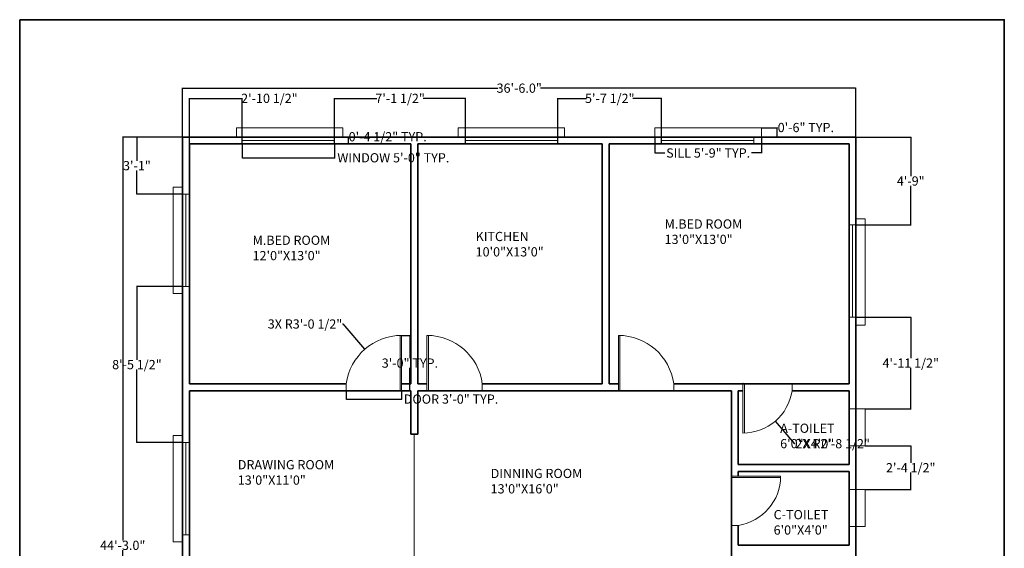
# Model space of a CAD drawing. Units: inches. Extents: x 2946 to 3586, y 7561 to 8235.
# Tile 2 of 2: x 2946 to 3586, y 7891 to 8235. Entities that reach past the tile are written whole.
import ezdxf

# ---------------------------------------------------------------- set-up
doc = ezdxf.new("R2010")
doc.units = ezdxf.units.IN
doc.header["$MEASUREMENT"] = 0
for name, color, linetype, lineweight in [('A-ANNO-DIMS', 2, 'Continuous', 18), ('A-ANNO-TTLB', 7, 'Continuous', 35), ('A-AREA-IDEN', 7, 'Continuous', 18), ('A-DOOR', 4, 'Continuous', 18), ('A-GLAZ-VENT', 130, 'Continuous', 18), ('A-WALL', 7, 'Continuous', 35), ('windows', 130, 'Continuous', 18)]:
    doc.layers.add(name, color=color, linetype=linetype, lineweight=lineweight)
doc.styles.get("Standard").update_dxf_attribs({"font": 'arial.ttf'})
doc.dimstyles.get("Standard").update_dxf_attribs({"dimtxt": 6, "dimasz": 0.18, "dimexe": 0.18, "dimexo": 0.0625, "dimgap": 0.09, "dimtad": 0, "dimtih": 1, "dimtoh": 1, "dimdec": 1, "dimzin": 0, "dimdsep": 46, "dimlunit": 3, "dimtxsty": 'Standard', "dimcen": 0.09, "dimadec": 0, "dimazin": 0, "dimtfac": 1, "dimtdec": 1, "dimtofl": 0, "dimtmove": 0, "dimatfit": 3, "dimfxl": 1, "dimtolj": 1, "dimtzin": 0, "dimarcsym": 0})

# ---------------------------------------------------------------- blocks, each defined once
blk = doc.blocks.new('*D1')
at = {"layer": 'A-ANNO-DIMS', "color": 0, "lineweight": -2, "transparency": 16777216}
for p, q in [((3051.51, 8158.52), (3051.51, 8190.42)), ((3051.69, 8190.24), (3256.62, 8190.24)), ((3489.33, 8190.24), (3284.4, 8190.24)), ((3489.51, 8158.52), (3489.51, 8190.42))]:
    blk.add_line(p, q, dxfattribs=at)
at = {"layer": 'A-ANNO-DIMS', "color": 0, "transparency": 16777216}
for points in [[(3051.69, 8190.27), (3051.69, 8190.21), (3051.51, 8190.24)], [(3489.33, 8190.27), (3489.33, 8190.21), (3489.51, 8190.24)]]:
    blk.add_solid(points, dxfattribs=at)
at = {"layer": 'Defpoints', "color": 0, "transparency": 16777216}
for p in [(3489.51, 8190.24), (3051.51, 8158.46), (3489.51, 8158.46)]:
    blk.add_point(p, dxfattribs=at)
at = {"layer": 'A-ANNO-DIMS', "color": 0, "transparency": 16777216, "insert": (3270.51, 8190.24), "char_height": 6, "width": 27.5975, "attachment_point": 5}
blk.add_mtext('\\A1;36\'-6.0"', dxfattribs=at)
blk = doc.blocks.new('*D2')
at = {"layer": 'A-ANNO-DIMS', "color": 0, "lineweight": -2, "transparency": 16777216}
for p, q in [((3051.44, 8158.46), (3012.47, 8158.46)), ((3012.65, 8158.28), (3012.65, 7896.12)), ((3012.65, 7627.64), (3012.65, 7889.81)), ((3051.44, 7627.46), (3012.47, 7627.46))]:
    blk.add_line(p, q, dxfattribs=at)
at = {"layer": 'A-ANNO-DIMS', "color": 0, "transparency": 16777216}
for points in [[(3012.62, 8158.28), (3012.68, 8158.28), (3012.65, 8158.46)], [(3012.62, 7627.64), (3012.68, 7627.64), (3012.65, 7627.46)]]:
    blk.add_solid(points, dxfattribs=at)
at = {"layer": 'Defpoints', "color": 0, "transparency": 16777216}
for p in [(3051.51, 8158.46), (3012.65, 7627.46), (3051.51, 7627.46)]:
    blk.add_point(p, dxfattribs=at)
at = {"layer": 'A-ANNO-DIMS', "color": 0, "transparency": 16777216, "insert": (3012.65, 7892.96), "char_height": 6, "attachment_point": 5}
blk.add_mtext('\\A1;44\'-3.0"', dxfattribs=at)
blk = doc.blocks.new('DOOR-SINGLE-36IN')
for p, q in [((-1, 36), (-1, 0)), ((0, 0), (0, 36)), ((0, 36), (0, 0)), ((-36, 0), (-36, 4.5)), ((0, 0), (-36, 0))]:
    blk.add_line(p, q)
blk.add_arc((0, -0.32), 36.32, 90, 172.37185)
blk = doc.blocks.new('DOOR-SINGLE-32IN')
for p, q in [((0, 0), (0, -32)), ((0, -32), (0, 0)), ((0, 0), (32, 0)), ((1, -32), (1, 0)), ((32, 0), (32, -4.5))]:
    blk.add_line(p, q)
blk.add_arc((0, 0.37), 32.37, 270, 351.34988)
blk = doc.blocks.new('WIN-60IN')
for p, q in [((0, 0), (0, -4.5)), ((60, 0), (0, 0)), ((0, -2.25), (60, -2.25)), ((0, -4.5), (60, -4.5)), ((60, -4.5), (60, 0))]:
    blk.add_line(p, q)
blk = doc.blocks.new('WIN-SILL-60IN')
for p, q in [((0, 0), (0, 6)), ((0, 6), (69.18, 6)), ((69.18, 6), (69.18, 0))]:
    blk.add_line(p, q)
blk = doc.blocks.new('VENT-24IN')
for p, q in [((0, 0), (4.5, 0)), ((0, -24), (0, 0)), ((4.5, 0), (4.5, -24)), ((4.5, 0), (10.5, 0)), ((10.5, 0), (10.5, -24)), ((4.5, -24), (0, -24)), ((10.5, -24), (4.5, -24))]:
    blk.add_line(p, q)
blk = doc.blocks.new('*D8')
at = {"layer": 'A-ANNO-DIMS', "color": 0, "lineweight": -2, "transparency": 16777216}
for p, q in [((3090.41, 8153.9), (3090.41, 8144.78)), ((3150.41, 8153.9), (3150.41, 8144.78)), ((3090.59, 8144.96), (3150.23, 8144.96)), ((3150.41, 8144.96), (3150.59, 8144.96))]:
    blk.add_line(p, q, dxfattribs=at)
at = {"layer": 'A-ANNO-DIMS', "color": 0, "transparency": 16777216}
for points in [[(3090.59, 8144.99), (3090.59, 8144.93), (3090.41, 8144.96)], [(3150.23, 8144.99), (3150.23, 8144.93), (3150.41, 8144.96)]]:
    blk.add_solid(points, dxfattribs=at)
at = {"layer": 'Defpoints', "color": 0, "transparency": 16777216}
for p in [(3090.41, 8153.96), (3150.41, 8153.96), (3150.41, 8144.96)]:
    blk.add_point(p, dxfattribs=at)
at = {"layer": 'A-ANNO-DIMS', "color": 0, "transparency": 16777216, "insert": (3188.64, 8144.96), "char_height": 6, "attachment_point": 5}
blk.add_mtext('\\A1;WINDOW 5\'-0" TYP.', dxfattribs=at)
blk = doc.blocks.new('*D9')
at = {"layer": 'A-ANNO-DIMS', "color": 0, "lineweight": -2, "transparency": 16777216}
for p, q in [((3159.41, 8158.46), (3159.41, 8158.64)), ((3159.41, 8158.64), (3159.59, 8158.64)), ((3150.47, 8158.46), (3159.59, 8158.46)), ((3150.47, 8153.96), (3159.59, 8153.96)), ((3159.41, 8154.14), (3159.41, 8158.28))]:
    blk.add_line(p, q, dxfattribs=at)
at = {"layer": 'A-ANNO-DIMS', "color": 0, "transparency": 16777216}
for points in [[(3159.38, 8158.28), (3159.44, 8158.28), (3159.41, 8158.46)], [(3159.38, 8154.14), (3159.44, 8154.14), (3159.41, 8153.96)]]:
    blk.add_solid(points, dxfattribs=at)
at = {"layer": 'Defpoints', "color": 0, "transparency": 16777216}
for p in [(3150.41, 8158.46), (3150.41, 8153.96), (3159.41, 8158.46)]:
    blk.add_point(p, dxfattribs=at)
at = {"layer": 'A-ANNO-DIMS', "color": 0, "transparency": 16777216, "insert": (3184.96, 8158.64), "char_height": 6, "attachment_point": 5}
blk.add_mtext('\\A1;0\'-4 1/2" TYP.', dxfattribs=at)
blk = doc.blocks.new('*D10')
at = {"layer": 'A-ANNO-DIMS', "color": 0, "lineweight": -2, "transparency": 16777216}
for p, q in [((3358.82, 8158.4), (3358.82, 8147.9)), ((3428, 8158.4), (3428, 8147.9)), ((3359, 8148.08), (3365.26, 8148.08)), ((3427.82, 8148.08), (3421.56, 8148.08))]:
    blk.add_line(p, q, dxfattribs=at)
at = {"layer": 'A-ANNO-DIMS', "color": 0, "transparency": 16777216}
for points in [[(3359, 8148.11), (3359, 8148.05), (3358.82, 8148.08)], [(3427.82, 8148.11), (3427.82, 8148.05), (3428, 8148.08)]]:
    blk.add_solid(points, dxfattribs=at)
at = {"layer": 'Defpoints', "color": 0, "transparency": 16777216}
for p in [(3358.82, 8158.46), (3428, 8158.46), (3428, 8148.08)]:
    blk.add_point(p, dxfattribs=at)
at = {"layer": 'A-ANNO-DIMS', "color": 0, "transparency": 16777216, "insert": (3393.41, 8148.08), "char_height": 6, "attachment_point": 5}
blk.add_mtext('\\A1;SILL 5\'-9" TYP.', dxfattribs=at)
blk = doc.blocks.new('*D11')
at = {"layer": 'A-ANNO-DIMS', "color": 0, "lineweight": -2, "transparency": 16777216}
for p, q in [((3428.06, 8164.46), (3438.56, 8164.46)), ((3438.38, 8164.46), (3438.38, 8164.64)), ((3438.38, 8164.64), (3438.56, 8164.64)), ((3438.38, 8158.64), (3438.38, 8164.28)), ((3428.06, 8158.46), (3438.56, 8158.46))]:
    blk.add_line(p, q, dxfattribs=at)
at = {"layer": 'A-ANNO-DIMS', "color": 0, "transparency": 16777216}
for points in [[(3438.35, 8164.28), (3438.41, 8164.28), (3438.38, 8164.46)], [(3438.35, 8158.64), (3438.41, 8158.64), (3438.38, 8158.46)]]:
    blk.add_solid(points, dxfattribs=at)
at = {"layer": 'Defpoints', "color": 0, "transparency": 16777216}
for p in [(3428, 8164.46), (3438.38, 8164.46), (3428, 8158.46)]:
    blk.add_point(p, dxfattribs=at)
at = {"layer": 'A-ANNO-DIMS', "color": 0, "transparency": 16777216, "insert": (3456.93, 8164.64), "char_height": 6, "attachment_point": 5}
blk.add_mtext('\\A1;0\'-6" TYP.', dxfattribs=at)
blk = doc.blocks.new('*D12')
at = {"layer": 'A-ANNO-DIMS', "color": 0, "lineweight": -2, "transparency": 16777216}
for p, q in [((3158.01, 7993.4), (3158.01, 7987.88)), ((3194.01, 7993.4), (3194.01, 7987.88)), ((3158.19, 7988.06), (3193.83, 7988.06)), ((3194.01, 7988.06), (3194.19, 7988.06))]:
    blk.add_line(p, q, dxfattribs=at)
at = {"layer": 'A-ANNO-DIMS', "color": 0, "transparency": 16777216}
for points in [[(3158.19, 7988.09), (3158.19, 7988.03), (3158.01, 7988.06)], [(3193.83, 7988.09), (3193.83, 7988.03), (3194.01, 7988.06)]]:
    blk.add_solid(points, dxfattribs=at)
at = {"layer": 'Defpoints', "color": 0, "transparency": 16777216}
for p in [(3158.01, 7993.46), (3194.01, 7993.46), (3194.01, 7988.06)]:
    blk.add_point(p, dxfattribs=at)
at = {"layer": 'A-ANNO-DIMS', "color": 0, "transparency": 16777216, "insert": (3226.15, 7988.06), "char_height": 6, "attachment_point": 5}
blk.add_mtext('\\A1;DOOR 3\'-0" TYP.', dxfattribs=at)
blk = doc.blocks.new('*D13')
at = {"layer": 'A-ANNO-DIMS', "color": 0, "lineweight": -2, "transparency": 16777216}
for p, q in [((3194.07, 8029.46), (3199.59, 8029.46)), ((3199.41, 8029.28), (3199.41, 8014.62)), ((3199.41, 7993.64), (3199.41, 8008.31)), ((3194.07, 7993.46), (3199.59, 7993.46))]:
    blk.add_line(p, q, dxfattribs=at)
at = {"layer": 'A-ANNO-DIMS', "color": 0, "transparency": 16777216}
for points in [[(3199.38, 8029.28), (3199.44, 8029.28), (3199.41, 8029.46)], [(3199.38, 7993.64), (3199.44, 7993.64), (3199.41, 7993.46)]]:
    blk.add_solid(points, dxfattribs=at)
at = {"layer": 'Defpoints', "color": 0, "transparency": 16777216}
for p in [(3194.01, 8029.46), (3199.41, 8029.46), (3194.01, 7993.46)]:
    blk.add_point(p, dxfattribs=at)
at = {"layer": 'A-ANNO-DIMS', "color": 0, "transparency": 16777216, "insert": (3199.41, 8011.46), "char_height": 6, "attachment_point": 5}
blk.add_mtext('\\A1;3\'-0" TYP.', dxfattribs=at)
blk = doc.blocks.new('*D17')
at = {"layer": 'A-ANNO-DIMS', "color": 0, "lineweight": -2, "transparency": 16777216}
for p, q in [((3485.01, 7875.79), (3485.01, 7879.51)), ((3485.19, 7879.33), (3495.33, 7879.33)), ((3495.51, 7875.79), (3495.51, 7879.51)), ((3495.51, 7879.33), (3495.69, 7879.33))]:
    blk.add_line(p, q, dxfattribs=at)
at = {"layer": 'A-ANNO-DIMS', "color": 0, "transparency": 16777216}
for points in [[(3485.19, 7879.36), (3485.19, 7879.3), (3485.01, 7879.33)], [(3495.33, 7879.36), (3495.33, 7879.3), (3495.51, 7879.33)]]:
    blk.add_solid(points, dxfattribs=at)
at = {"layer": 'Defpoints', "color": 0, "transparency": 16777216}
for p in [(3495.51, 7879.33), (3485.01, 7875.73), (3495.51, 7875.73)]:
    blk.add_point(p, dxfattribs=at)
at = {"layer": 'A-ANNO-DIMS', "color": 0, "transparency": 16777216, "insert": (3523.39, 7879.33), "char_height": 6, "attachment_point": 5}
blk.add_mtext('\\A1;0\'-10 1/2" TYP.', dxfattribs=at)
blk = doc.blocks.new('*D18')
at = {"layer": 'A-ANNO-DIMS', "color": 0, "lineweight": -2, "transparency": 16777216}
for p, q in [((3056.01, 8154.02), (3056.01, 8183.79)), ((3056.19, 8183.61), (3090.23, 8183.61)), ((3090.41, 8154.02), (3090.41, 8183.79)), ((3090.41, 8183.61), (3090.59, 8183.61))]:
    blk.add_line(p, q, dxfattribs=at)
at = {"layer": 'A-ANNO-DIMS', "color": 0, "transparency": 16777216}
for points in [[(3056.19, 8183.64), (3056.19, 8183.58), (3056.01, 8183.61)], [(3090.23, 8183.64), (3090.23, 8183.58), (3090.41, 8183.61)]]:
    blk.add_solid(points, dxfattribs=at)
at = {"layer": 'Defpoints', "color": 0, "transparency": 16777216}
for p in [(3090.41, 8183.61), (3056.01, 8153.96), (3090.41, 8153.96)]:
    blk.add_point(p, dxfattribs=at)
at = {"layer": 'A-ANNO-DIMS', "color": 0, "transparency": 16777216, "insert": (3108.03, 8183.61), "char_height": 6, "attachment_point": 5}
blk.add_mtext('\\A1;2\'-10 1/2"', dxfattribs=at)
blk = doc.blocks.new('*D19')
at = {"layer": 'A-ANNO-DIMS', "color": 0, "lineweight": -2, "transparency": 16777216}
for p, q in [((3150.41, 8154.02), (3150.41, 8183.79)), ((3150.59, 8183.61), (3178.01, 8183.61)), ((3235.49, 8183.61), (3208.07, 8183.61)), ((3235.67, 8154.02), (3235.67, 8183.79))]:
    blk.add_line(p, q, dxfattribs=at)
at = {"layer": 'A-ANNO-DIMS', "color": 0, "transparency": 16777216}
for points in [[(3150.59, 8183.64), (3150.59, 8183.58), (3150.41, 8183.61)], [(3235.49, 8183.64), (3235.49, 8183.58), (3235.67, 8183.61)]]:
    blk.add_solid(points, dxfattribs=at)
at = {"layer": 'Defpoints', "color": 0, "transparency": 16777216}
for p in [(3235.67, 8183.61), (3150.41, 8153.96), (3235.67, 8153.96)]:
    blk.add_point(p, dxfattribs=at)
at = {"layer": 'A-ANNO-DIMS', "color": 0, "transparency": 16777216, "insert": (3193.04, 8183.61), "char_height": 6, "attachment_point": 5}
blk.add_mtext('\\A1;7\'-1 1/2"', dxfattribs=at)
blk = doc.blocks.new('*D20')
at = {"layer": 'A-ANNO-DIMS', "color": 0, "lineweight": -2, "transparency": 16777216}
for p, q in [((3295.67, 8154.02), (3295.67, 8183.79)), ((3295.85, 8183.61), (3314.36, 8183.61)), ((3362.97, 8183.61), (3344.47, 8183.61)), ((3363.15, 8154.02), (3363.15, 8183.79))]:
    blk.add_line(p, q, dxfattribs=at)
at = {"layer": 'A-ANNO-DIMS', "color": 0, "transparency": 16777216}
for points in [[(3295.85, 8183.64), (3295.85, 8183.58), (3295.67, 8183.61)], [(3362.97, 8183.64), (3362.97, 8183.58), (3363.15, 8183.61)]]:
    blk.add_solid(points, dxfattribs=at)
at = {"layer": 'Defpoints', "color": 0, "transparency": 16777216}
for p in [(3363.15, 8183.61), (3295.67, 8153.96), (3363.15, 8153.96)]:
    blk.add_point(p, dxfattribs=at)
at = {"layer": 'A-ANNO-DIMS', "color": 0, "transparency": 16777216, "insert": (3329.41, 8183.61), "char_height": 6, "attachment_point": 5}
blk.add_mtext('\\A1;5\'-7 1/2"', dxfattribs=at)
blk = doc.blocks.new('*D21')
at = {"layer": 'A-ANNO-DIMS', "color": 0, "lineweight": -2, "transparency": 16777216}
for p, q in [((3051.44, 8158.46), (3021.68, 8158.46)), ((3021.86, 8158.28), (3021.86, 8143.01)), ((3021.86, 8121.43), (3021.86, 8136.7)), ((3051.44, 8121.25), (3021.68, 8121.25))]:
    blk.add_line(p, q, dxfattribs=at)
at = {"layer": 'A-ANNO-DIMS', "color": 0, "transparency": 16777216}
for points in [[(3021.83, 8158.28), (3021.89, 8158.28), (3021.86, 8158.46)], [(3021.83, 8121.43), (3021.89, 8121.43), (3021.86, 8121.25)]]:
    blk.add_solid(points, dxfattribs=at)
at = {"layer": 'Defpoints', "color": 0, "transparency": 16777216}
for p in [(3021.86, 8158.46), (3051.51, 8158.46), (3051.51, 8121.25)]:
    blk.add_point(p, dxfattribs=at)
at = {"layer": 'A-ANNO-DIMS', "color": 0, "transparency": 16777216, "insert": (3021.86, 8139.85), "char_height": 6, "attachment_point": 5}
blk.add_mtext('\\A1;3\'-1"', dxfattribs=at)
blk = doc.blocks.new('*D22')
at = {"layer": 'A-ANNO-DIMS', "color": 0, "lineweight": -2, "transparency": 16777216}
for p, q in [((3051.44, 8061.25), (3021.68, 8061.25)), ((3021.86, 8061.07), (3021.86, 8013.68)), ((3021.86, 7959.91), (3021.86, 8007.29)), ((3051.44, 7959.73), (3021.68, 7959.73))]:
    blk.add_line(p, q, dxfattribs=at)
at = {"layer": 'A-ANNO-DIMS', "color": 0, "transparency": 16777216}
for points in [[(3021.83, 8061.07), (3021.89, 8061.07), (3021.86, 8061.25)], [(3021.83, 7959.91), (3021.89, 7959.91), (3021.86, 7959.73)]]:
    blk.add_solid(points, dxfattribs=at)
at = {"layer": 'Defpoints', "color": 0, "transparency": 16777216}
for p in [(3021.86, 8061.25), (3051.51, 8061.25), (3051.51, 7959.73)]:
    blk.add_point(p, dxfattribs=at)
at = {"layer": 'A-ANNO-DIMS', "color": 0, "transparency": 16777216, "insert": (3021.86, 8010.49), "char_height": 6, "attachment_point": 5}
blk.add_mtext('\\A1;8\'-5 1/2"', dxfattribs=at)
blk = doc.blocks.new('*D23')
at = {"layer": 'A-ANNO-DIMS', "color": 0, "lineweight": -2, "transparency": 16777216}
for p, q in [((3489.57, 8158.46), (3525.34, 8158.46)), ((3525.16, 8158.28), (3525.16, 8133.01)), ((3525.16, 8101.44), (3525.16, 8126.71)), ((3489.57, 8101.26), (3525.34, 8101.26))]:
    blk.add_line(p, q, dxfattribs=at)
at = {"layer": 'A-ANNO-DIMS', "color": 0, "transparency": 16777216}
for points in [[(3525.13, 8158.28), (3525.19, 8158.28), (3525.16, 8158.46)], [(3525.13, 8101.44), (3525.19, 8101.44), (3525.16, 8101.26)]]:
    blk.add_solid(points, dxfattribs=at)
at = {"layer": 'Defpoints', "color": 0, "transparency": 16777216}
for p in [(3489.51, 8158.46), (3525.16, 8158.46), (3489.51, 8101.26)]:
    blk.add_point(p, dxfattribs=at)
at = {"layer": 'A-ANNO-DIMS', "color": 0, "transparency": 16777216, "insert": (3525.16, 8129.86), "char_height": 6, "attachment_point": 5}
blk.add_mtext('\\A1;4\'-9"', dxfattribs=at)
blk = doc.blocks.new('*D24')
at = {"layer": 'A-ANNO-DIMS', "color": 0, "lineweight": -2, "transparency": 16777216}
for p, q in [((3489.57, 8041.26), (3525.34, 8041.26)), ((3525.16, 8041.08), (3525.16, 8014.66)), ((3525.16, 7981.87), (3525.16, 8008.28)), ((3495.57, 7981.69), (3525.34, 7981.69))]:
    blk.add_line(p, q, dxfattribs=at)
at = {"layer": 'A-ANNO-DIMS', "color": 0, "transparency": 16777216}
for points in [[(3525.13, 8041.08), (3525.19, 8041.08), (3525.16, 8041.26)], [(3525.13, 7981.87), (3525.19, 7981.87), (3525.16, 7981.69)]]:
    blk.add_solid(points, dxfattribs=at)
at = {"layer": 'Defpoints', "color": 0, "transparency": 16777216}
for p in [(3489.51, 8041.26), (3525.16, 8041.26), (3495.51, 7981.69)]:
    blk.add_point(p, dxfattribs=at)
at = {"layer": 'A-ANNO-DIMS', "color": 0, "transparency": 16777216, "insert": (3525.16, 8011.47), "char_height": 6, "attachment_point": 5}
blk.add_mtext('\\A1;4\'-11 1/2"', dxfattribs=at)
blk = doc.blocks.new('*D25')
at = {"layer": 'A-ANNO-DIMS', "color": 0, "lineweight": -2, "transparency": 16777216}
for p, q in [((3495.57, 7957.69), (3525.34, 7957.69)), ((3525.16, 7957.51), (3525.16, 7946.62)), ((3525.16, 7929.35), (3525.16, 7940.23)), ((3495.57, 7929.17), (3525.34, 7929.17))]:
    blk.add_line(p, q, dxfattribs=at)
at = {"layer": 'A-ANNO-DIMS', "color": 0, "transparency": 16777216}
for points in [[(3525.13, 7957.51), (3525.19, 7957.51), (3525.16, 7957.69)], [(3525.13, 7929.35), (3525.19, 7929.35), (3525.16, 7929.17)]]:
    blk.add_solid(points, dxfattribs=at)
at = {"layer": 'Defpoints', "color": 0, "transparency": 16777216}
for p in [(3495.51, 7957.69), (3525.16, 7957.69), (3495.51, 7929.17)]:
    blk.add_point(p, dxfattribs=at)
at = {"layer": 'A-ANNO-DIMS', "color": 0, "transparency": 16777216, "insert": (3525.16, 7943.43), "char_height": 6, "attachment_point": 5}
blk.add_mtext('\\A1;2\'-4 1/2"', dxfattribs=at)
blk = doc.blocks.new('*D35')
at = {"layer": 'A-ANNO-DIMS', "color": 0, "lineweight": -2, "transparency": 16777216}
for p, q in [((3155.56, 8036.88), (3155.74, 8036.88)), ((3155.74, 8036.88), (3169.97, 8020.61)), ((3193.92, 7993.14), (3194.1, 7993.14)), ((3194.01, 7993.05), (3194.01, 7993.23))]:
    blk.add_line(p, q, dxfattribs=at)
at = {"layer": 'A-ANNO-DIMS', "color": 0, "transparency": 16777216}
blk.add_solid([(3169.99, 8020.63), (3169.95, 8020.59), (3170.09, 8020.48)], dxfattribs=at)
at = {"layer": 'Defpoints', "color": 0, "transparency": 16777216}
for p in [(3170.09, 8020.48), (3194.01, 7993.14)]:
    blk.add_point(p, dxfattribs=at)
at = {"layer": 'A-ANNO-DIMS', "color": 0, "transparency": 16777216, "insert": (3131.19, 8036.88), "char_height": 6, "attachment_point": 5}
blk.add_mtext('\\A1;3X R3\'-0 1/2"', dxfattribs=at)
blk = doc.blocks.new('*D36')
at = {"layer": 'A-ANNO-DIMS', "color": 0, "lineweight": -2, "transparency": 16777216}
for p, q in [((3415.92, 7998.33), (3416.1, 7998.33)), ((3416.01, 7998.24), (3416.01, 7998.42)), ((3449.76, 7959.05), (3437.22, 7973.64)), ((3449.94, 7959.05), (3449.76, 7959.05))]:
    blk.add_line(p, q, dxfattribs=at)
at = {"layer": 'A-ANNO-DIMS', "color": 0, "transparency": 16777216}
blk.add_solid([(3437.24, 7973.66), (3437.2, 7973.63), (3437.1, 7973.78)], dxfattribs=at)
at = {"layer": 'Defpoints', "color": 0, "transparency": 16777216}
for p in [(3416.01, 7998.33), (3437.1, 7973.78)]:
    blk.add_point(p, dxfattribs=at)
at = {"layer": 'A-ANNO-DIMS', "color": 0, "transparency": 16777216, "insert": (3474.37, 7959.05), "char_height": 6, "attachment_point": 5}
blk.add_mtext('\\A1;2X R2\'-8 1/2"', dxfattribs=at)

msp = doc.modelspace()

# ---------------------------------------------------------------- linework, layer by layer
at = {"layer": 'A-ANNO-TTLB'}
msp.add_lwpolyline([(2945.62, 8234.75), (3586.02, 8234.75), (3586.02, 7560.83), (2945.62, 7560.83)], close=True, dxfattribs=at)
at = {"layer": 'A-GLAZ-VENT'}
for p, q in [((3485.01, 7981.69), (3489.51, 7981.69)), ((3485.01, 7957.69), (3485.01, 7981.69)), ((3489.51, 7981.69), (3489.51, 7957.69)), ((3489.51, 7981.69), (3495.51, 7981.69)), ((3495.51, 7981.69), (3495.51, 7957.69)), ((3489.51, 7957.69), (3485.01, 7957.69)), ((3495.51, 7957.69), (3487.26, 7957.69))]:
    msp.add_line(p, q, dxfattribs=at)
at = {"layer": 'A-WALL'}
for p, q in [((3051.51, 8158.46), (3051.51, 7627.46)), ((3051.51, 8158.46), (3489.51, 8158.46)), ((3056.01, 8153.96), (3056.01, 7997.96)), ((3056.01, 8153.96), (3200.01, 8153.96)), ((3200.01, 8153.96), (3200.01, 7997.96)), ((3204.51, 8153.96), (3204.51, 7997.96)), ((3204.51, 8153.96), (3324.51, 8153.96)), ((3324.51, 8153.96), (3324.51, 7997.96)), ((3329.01, 8153.96), (3329.01, 7997.96)), ((3329.01, 8153.96), (3485.01, 8153.96)), ((3485.01, 8153.96), (3485.01, 7997.96)), ((3489.51, 8158.46), (3489.51, 7627.46)), ((3056.01, 7997.96), (3158.01, 7997.96)), ((3056.01, 7993.46), (3200.01, 7993.46)), ((3056.01, 7993.46), (3056.01, 7840.46)), ((3194.01, 7997.96), (3200.01, 7997.96)), ((3200.01, 7993.46), (3194.01, 7993.46)), ((3200.01, 7993.46), (3200.01, 7965.14)), ((3204.51, 7997.96), (3210.51, 7997.96)), ((3204.51, 7993.46), (3210.51, 7993.46)), ((3204.51, 7993.46), (3204.51, 7965.14)), ((3204.51, 7993.46), (3408.51, 7993.46)), ((3246.51, 7997.96), (3324.51, 7997.96)), ((3329.01, 7997.96), (3335.01, 7997.96)), ((3329.01, 7993.46), (3335.01, 7993.46)), ((3371.01, 7997.96), (3485.01, 7997.96)), ((3408.51, 7993.46), (3408.51, 7840.46)), ((3413.01, 7997.96), (3416.01, 7997.96)), ((3413.01, 7993.46), (3413.01, 7945.46)), ((3413.01, 7993.46), (3416.01, 7993.46)), ((3448.01, 7993.46), (3485.01, 7993.46)), ((3485.01, 7993.46), (3485.01, 7945.46)), ((3200.01, 7965.14), (3204.51, 7965.14)), ((3408.51, 7940.96), (3408.51, 7937.96)), ((3413.01, 7945.46), (3485.01, 7945.46)), ((3413.01, 7940.96), (3485.01, 7940.96)), ((3413.01, 7940.96), (3413.01, 7937.96)), ((3485.01, 7940.96), (3485.01, 7892.96)), ((3413.01, 7905.96), (3413.01, 7892.96)), ((3413.01, 7892.96), (3485.01, 7892.96))]:
    msp.add_line(p, q, dxfattribs=at)
at = {"layer": 'windows'}
for p, q in [((3485.01, 8041.26), (3485.01, 8041.26)), ((3202.26, 7965.14), (3202.26, 7877.43))]:
    msp.add_line(p, q, dxfattribs=at)

# ---------------------------------------------------------------- block references
at = {"layer": 'A-DOOR'}
for name, p in [('DOOR-SINGLE-36IN', (3194.01, 7993.46)), ('DOOR-SINGLE-32IN', (3416.01, 7997.96))]:
    msp.add_blockref(name, p, dxfattribs=at)
at = {"layer": 'A-DOOR', "extrusion": (0, 0, -1), "zscale": -1}
for p in [(-3210.51, 7993.46), (-3335.01, 7993.46)]:
    msp.add_blockref('DOOR-SINGLE-36IN', p, dxfattribs=at)
at = {"layer": 'A-DOOR', "extrusion": (0, 0, -1), "zscale": -1, "rotation": 270.0000000000025}
msp.add_blockref('DOOR-SINGLE-32IN', (-3408.51, 7937.96), dxfattribs=at)
at = {"layer": 'A-GLAZ-VENT'}
msp.add_blockref('VENT-24IN', (3485.01, 7929.17), dxfattribs=at)
at = {"layer": 'windows'}
for name, p in [('WIN-SILL-60IN', (3086.66, 8158.46)), ('WIN-SILL-60IN', (3230.81, 8158.46)), ('WIN-SILL-60IN', (3358.82, 8158.46)), ('WIN-60IN', (3090.41, 8158.46))]:
    msp.add_blockref(name, p, dxfattribs=at)
for name, p, rotation in [('WIN-60IN', (3295.67, 8153.96), 180), ('WIN-60IN', (3423.15, 8153.96), 180), ('WIN-SILL-60IN', (3051.51, 8056.71), 89.99999999999984), ('WIN-60IN', (3051.51, 8061.25), 90.00000000000325), ('WIN-60IN', (3485.01, 8041.26), 90.000000000004), ('WIN-SILL-60IN', (3489.51, 8105.31), 270), ('WIN-SILL-60IN', (3051.51, 7895.17), 90.00000000000033), ('WIN-60IN', (3051.51, 7899.73), 90.000000000003)]:
    msp.add_blockref(name, p, dxfattribs=dict(at, rotation=rotation))

# ---------------------------------------------------------------- texts
at = {"layer": 'A-AREA-IDEN', "char_height": 6, "attachment_point": 1}
for s, width, insert in [('M.BED ROOM\\P13\'0"X13\'0"', 97.6416, (3365.07, 8104.91)), ('KITCHEN\\P10\'0"X13\'0"', 73.4039, (3242.16, 8096.8)), ('M.BED ROOM\\P12\'0"X13\'0"', 91.3548, (3097.1, 8094.35)), ('A-TOILET\\P6\'0"X4\'0"', 38.2975, (3440.24, 7972.1)), ('DRAWING ROOM\\P13\'0"X11\'0"', 96.5054, (3087.46, 7948.38)), ('DINNING ROOM\\P13\'0"X16\'0"', 123.1277, (3251.93, 7942.7)), ('C-TOILET\\P6\'0"X4\'0"', 41.074, (3435.99, 7915.92))]:
    msp.add_mtext_dynamic_manual_height_columns(s, width=width, gutter_width=1, heights=[0], dxfattribs=dict(at, insert=insert))

# ---------------------------------------------------------------- dimensions: what is measured, and where the dimension line sits
at = {"layer": 'A-ANNO-DIMS'}
for base, p1, p2, override, picture, middle in [((3489.51, 8190.24), (3051.51, 8158.46), (3489.51, 8158.46), {"dimclrd": 0, "dimclre": 0, "dimclrt": 0}, '*D1', (3270.51, 8190.24)), ((3090.41, 8183.61), (3056.01, 8153.96), (3090.41, 8153.96), {"dimdec": 1, "dimlfac": 1, "dimrnd": 0, "dimzin": 1, "dimdsep": 46, "dimlunit": 4, "dimfrac": 2}, '*D18', (3108.03, 8183.61)), ((3363.15, 8183.61), (3295.67, 8153.96), (3363.15, 8153.96), {"dimdec": 1, "dimlfac": 1, "dimrnd": 0, "dimzin": 1, "dimdsep": 46, "dimlunit": 4, "dimfrac": 2}, '*D20', (3329.41, 8183.61))]:
    dim = msp.add_linear_dim(base=base, p1=p1, p2=p2, dimstyle='Standard', override=override, dxfattribs=at)
    dim.commit()
    dim.dimension.update_dxf_attribs({"geometry": picture, "text_midpoint": middle})
for base, p1, p2, angle, override, picture, middle in [((3235.67, 8183.61), (3150.41, 8153.96), (3235.67, 8153.96), 0, {"dimdec": 1, "dimlfac": 1, "dimrnd": 0, "dimzin": 1, "dimdsep": 46, "dimlunit": 4, "dimfrac": 2}, '*D19', (3193.04, 8183.61)), ((3012.65, 7627.46), (3051.51, 8158.46), (3051.51, 7627.46), 90, {"dimclrd": 0, "dimclre": 0, "dimclrt": 0}, '*D2', (3012.65, 7892.96)), ((3021.86, 8158.46), (3051.51, 8121.25), (3051.51, 8158.46), 90, {"dimdec": 1, "dimlfac": 1, "dimrnd": 0, "dimzin": 1, "dimdsep": 46, "dimlunit": 4, "dimfrac": 2}, '*D21', (3021.86, 8139.85)), ((3525.16, 8158.46), (3489.51, 8101.26), (3489.51, 8158.46), 90, {"dimdec": 1, "dimlfac": 1, "dimrnd": 0, "dimzin": 1, "dimdsep": 46, "dimlunit": 4, "dimfrac": 2}, '*D23', (3525.16, 8129.86)), ((3021.86, 8061.25), (3051.51, 7959.73), (3051.51, 8061.25), 90, {"dimdec": 1, "dimlfac": 1, "dimrnd": 0, "dimzin": 1, "dimdsep": 46, "dimlunit": 4, "dimfrac": 2}, '*D22', (3021.86, 8010.49)), ((3525.16, 8041.26), (3495.51, 7981.69), (3489.51, 8041.26), 90, {"dimdec": 1, "dimlfac": 1, "dimrnd": 0, "dimzin": 1, "dimdsep": 46, "dimlunit": 4, "dimfrac": 2}, '*D24', (3525.16, 8011.47)), ((3525.16, 7957.69), (3495.51, 7929.17), (3495.51, 7957.69), 90, {"dimdec": 1, "dimlfac": 1, "dimrnd": 0, "dimzin": 1, "dimdsep": 46, "dimlunit": 4, "dimfrac": 2}, '*D25', (3525.16, 7943.43))]:
    dim = msp.add_linear_dim(base=base, p1=p1, p2=p2, angle=angle, dimstyle='Standard', override=override, dxfattribs=at)
    dim.commit()
    dim.dimension.update_dxf_attribs({"geometry": picture, "text_midpoint": middle})
for base, p1, p2, picture, middle in [((3159.41, 8158.46), (3150.41, 8153.96), (3150.41, 8158.46), '*D9', (3184.96, 8158.64)), ((3438.38, 8164.46), (3428, 8158.46), (3428, 8164.46), '*D11', (3456.93, 8164.64)), ((3199.41, 8029.46), (3194.01, 7993.46), (3194.01, 8029.46), '*D13', (3199.41, 8011.46))]:
    dim = msp.add_linear_dim(base=base, p1=p1, p2=p2, angle=90, text='<> TYP.', dimstyle='Standard', override={"dimdec": 1, "dimlfac": 1, "dimrnd": 0, "dimzin": 1, "dimdsep": 46, "dimlunit": 4, "dimfrac": 2}, dxfattribs=at)
    dim.commit()
    dim.dimension.update_dxf_attribs({"geometry": picture, "text_midpoint": middle})
for base, p1, p2, text, picture, middle in [((3150.41, 8144.96), (3090.41, 8153.96), (3150.41, 8153.96), 'WINDOW <> TYP.', '*D8', (3188.64, 8144.96)), ((3428, 8148.08), (3358.82, 8158.46), (3428, 8158.46), 'SILL <> TYP.', '*D10', (3393.41, 8148.08)), ((3194.01, 7988.06), (3158.01, 7993.46), (3194.01, 7993.46), 'DOOR <> TYP.', '*D12', (3226.15, 7988.06)), ((3495.51, 7879.33), (3485.01, 7875.73), (3495.51, 7875.73), '<> TYP.', '*D17', (3523.39, 7879.33))]:
    dim = msp.add_linear_dim(base=base, p1=p1, p2=p2, text=text, dimstyle='Standard', override={"dimdec": 1, "dimlfac": 1, "dimrnd": 0, "dimzin": 1, "dimdsep": 46, "dimlunit": 4, "dimfrac": 2}, dxfattribs=at)
    dim.commit()
    dim.dimension.update_dxf_attribs({"geometry": picture, "text_midpoint": middle})
for center, mpoint, text, picture, middle in [((3194.01, 7993.14), (3170.09, 8020.48), '3X <>', '*D35', (3131.19, 8036.88)), ((3416.01, 7998.33), (3437.1, 7973.78), '2X <>', '*D36', (3474.37, 7959.05))]:
    dim = msp.add_radius_dim(center=center, mpoint=mpoint, text=text, dimstyle='Standard', override={"dimdec": 1, "dimlfac": 1, "dimrnd": 0, "dimzin": 1, "dimdsep": 46, "dimlunit": 4, "dimfrac": 2}, dxfattribs=at)
    dim.commit()
    dim.dimension.update_dxf_attribs({"geometry": picture, "text_midpoint": middle, "dimtype": 164})

doc.saveas('drawing.dxf')
